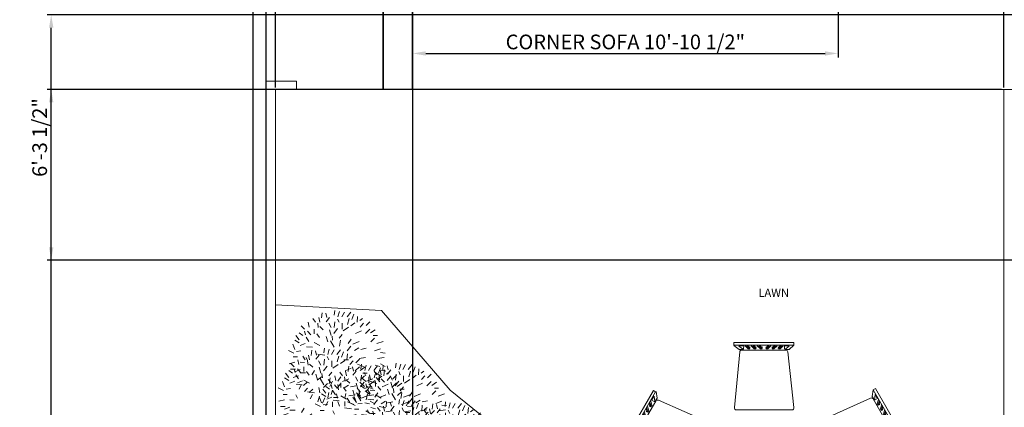
# Model space of a CAD drawing. Units: inches. Extents: x 1239 to 2276906, y 2273 to 321338.
# Tile 5 of 23: x 1239 to 1541, y 2510 to 2629. Entities that reach past the tile are written whole.
import ezdxf

# ---------------------------------------------------------------- set-up
doc = ezdxf.new("R2010")
doc.units = ezdxf.units.IN
for name, color, linetype, lineweight in [('A-ANNO-DIMS', 2, 'Continuous', 18), ('A-AREA-IDEN', 7, 'Continuous', 18), ('A-FURN', 8, 'Continuous', 13), ('C-PROP', 7, 'Continuous', 25), ('L-PLNT', 94, 'Continuous', 13), ('wall', 7, 'Continuous', 35)]:
    doc.layers.add(name, color=color, linetype=linetype, lineweight=lineweight)
doc.styles.get("Standard").update_dxf_attribs({"font": 'arial.ttf'})
doc.dimstyles.new('ISO-25', dxfattribs={"dimtxt": 4.5, "dimasz": 4, "dimexe": 1.25, "dimexo": 0.625, "dimtad": 1, "dimdec": 1, "dimlunit": 3, "dimtxsty": 'Standard', "dimcen": 2.5, "dimadec": 0, "dimazin": 0, "dimtfac": 1, "dimtdec": 1, "dimtmove": 0, "dimatfit": 3, "dimfxl": 1, "dimarcsym": 0})

# ---------------------------------------------------------------- blocks, each defined once
blk = doc.blocks.new('A$C20C17E7E')
for p, q in [((1.807, 4.871), (1.746, 5.147)), ((1.899, 5.117), (1.929, 5.423)), ((2.205, 5.147), (2.144, 5.393)), ((2.174, 4.903), (2.359, 5.147)), ((2.635, 5.271), (2.665, 5.546)), ((2.849, 5.179), (2.941, 5.485)), ((3.063, 5.179), (3.217, 5.455)), ((3.37, 5.179), (3.584, 5.455)), ((3.646, 5.025), (3.768, 5.332)), ((3.952, 4.871), (3.983, 5.21)), ((0.919, 4.474), (0.735, 4.658)), ((1.195, 4.597), (1.134, 4.871)), ((1.562, 4.871), (1.409, 5.086)), ((1.716, 4.565), (1.685, 4.81)), ((1.991, 4.443), (1.807, 4.627)), ((2.45, 4.565), (2.328, 4.81)), ((2.635, 4.565), (2.665, 4.903)), ((2.91, 4.871), (2.819, 5.056)), ((3.095, 4.474), (3.095, 4.81)), ((3.156, 4.382), (3.462, 4.597)), ((3.401, 4.749), (3.492, 5.086)), ((3.584, 4.658), (3.829, 4.841)), ((4.105, 4.964), (4.259, 5.086)), ((4.135, 4.597), (4.32, 4.81)), ((4.472, 4.688), (4.687, 4.903)), ((0.613, 3.861), (0.428, 4.106)), ((0.827, 4.106), (0.613, 4.259)), ((0.98, 4.137), (0.919, 4.352)), ((1.164, 3.77), (1.01, 4.014)), ((1.286, 4.137), (1.102, 4.352)), ((1.47, 4.198), (1.47, 4.474)), ((1.777, 3.983), (1.623, 4.198)), ((2.267, 3.739), (2.174, 4.045)), ((2.45, 4.106), (2.359, 4.443)), ((2.543, 3.831), (2.513, 4.076)), ((2.604, 4.228), (2.819, 4.504)), ((2.91, 3.953), (3.095, 4.167)), ((3.86, 4.228), (4.196, 4.382)), ((4.442, 4.228), (4.687, 4.474)), ((4.717, 4.259), (4.993, 4.443)), ((4.871, 4.106), (5.117, 4.106)), ((0.367, 3.31), (0.244, 3.616)), ((0.613, 3.677), (0.367, 3.831)), ((0.949, 3.646), (0.674, 3.524)), ((1.378, 3.431), (1.041, 3.463)), ((1.807, 3.524), (1.47, 3.707)), ((2.635, 3.431), (2.42, 3.8)), ((2.941, 3.494), (3.002, 3.831)), ((3.37, 3.218), (3.584, 3.494)), ((3.431, 3.646), (3.614, 3.892)), ((3.707, 3.616), (4.074, 3.77)), ((4.748, 3.739), (4.963, 3.953)), ((5.086, 3.646), (5.453, 3.77)), ((0.306, 3.095), (0, 3.249)), ((0.52, 2.88), (0.276, 2.88)), ((0.704, 3.218), (0.459, 3.188)), ((1.102, 2.666), (1.01, 2.849)), ((2.083, 2.973), (1.685, 3.034)), ((3.799, 3.249), (4.044, 3.401)), ((4.074, 2.788), (4.442, 2.849)), ((4.166, 3.31), (4.472, 3.37)), ((4.963, 3.218), (5.3, 3.34)), ((5.117, 2.788), (5.514, 2.849)), ((5.3, 3.125), (5.575, 3.095)), ((0.367, 2.574), (0.03, 2.482)), ((0.919, 2.543), (0.674, 2.574)), ((3.186, 2.697), (3.462, 2.697)), ((3.983, 2.452), (4.35, 2.298)), ((4.993, 2.391), (5.269, 2.33)), ((5.3, 2.482), (5.575, 2.33)), ((0.398, 2.176), (0.122, 2.176)), ((0.582, 1.778), (0.276, 1.685)), ((0.674, 2.145), (0.367, 2.022)), ((0.98, 1.961), (0.674, 1.961)), ((1.501, 2.084), (1.347, 1.839)), ((1.929, 1.748), (1.653, 1.533)), ((5.056, 1.931), (5.3, 1.778)), ((5.331, 2.115), (5.607, 2.054)), ((0.796, 1.502), (0.52, 1.379)), ((0.735, 1.257), (0.613, 1.012)), ((1.071, 1.409), (0.858, 1.226)), ((2.237, 1.348), (2.022, 1.103)), ((2.543, 1.472), (2.389, 1.164)), ((2.849, 1.287), (2.88, 0.981)), ((4.105, 1.409), (4.381, 1.164)), ((4.535, 1.164), (4.871, 1.012)), ((4.687, 1.472), (5.086, 1.348)), ((5.056, 1.685), (5.269, 1.44)), ((1.102, 1.073), (0.919, 0.888)), ((1.409, 1.012), (1.195, 0.827)), ((1.378, 0.705), (1.256, 0.46)), ((1.777, 0.614), (1.685, 0.276)), ((1.746, 1.103), (1.807, 0.797)), ((2.328, 0.827), (2.267, 0.521)), ((2.543, 0.951), (2.45, 0.705)), ((2.757, 0.736), (2.819, 0.491)), ((3.308, 0.766), (3.247, 0.491)), ((4.013, 0.736), (4.166, 0.491)), ((4.411, 0.92), (4.687, 0.705)), ((2.083, 0.521), (1.961, 0.215)), ((2.267, 0.306), (2.144, 0.062)), ((2.543, 0.276), (2.543, 0)), ((2.849, 0.306), (2.941, 0.03)), ((3.247, 0.306), (3.247, 0.03)), ((3.37, 0.491), (3.523, 0.245)), ((3.707, 0.552), (3.922, 0.245))]:
    blk.add_line(p, q)
blk = doc.blocks.new('A$C45501D90')
for p, q in [((-242.2, 1133.5), (224, 1133.5)), ((-242.2, 1112.8), (-242.2, 1133.5)), ((224, 1112.8), (-242.2, 1112.8)), ((-242.2, 1111.2), (-202.3, 1079.2)), ((-203.9, 1106.4), (-165.6, 1108)), ((-168.8, 1080.8), (-203.9, 1106.4)), ((-202.3, 1079.2), (-168.8, 1080.8)), ((161.8, 1076.1), (-181.4, 1076.1)), ((-165.6, 1108), (-167.2, 1085.6)), ((-156, 1109.6), (-132, 1085.6)), ((-119.3, 1085.6), (-143.2, 1108)), ((-143.2, 1108), (-133.6, 1108)), ((-133.6, 1108), (-122.5, 1098.4)), ((-132, 1085.6), (-119.3, 1085.6)), ((-122.5, 1098.4), (-119.3, 1101.6)), ((-119.3, 1101.6), (-117.7, 1087.2)), ((-108.1, 1109.6), (-84.1, 1085.6)), ((-71.4, 1085.6), (-95.3, 1108)), ((-95.3, 1108), (-85.7, 1108)), ((-85.7, 1108), (-74.6, 1098.4)), ((-84.1, 1085.6), (-71.4, 1085.6)), ((-74.6, 1098.4), (-71.4, 1101.6)), ((-71.4, 1101.6), (-69.8, 1087.2)), ((-60.2, 1109.6), (-36.2, 1085.6)), ((-23.5, 1085.6), (-47.4, 1108)), ((-47.4, 1108), (-37.8, 1108)), ((-37.8, 1108), (-26.7, 1098.4)), ((-36.2, 1085.6), (-23.5, 1085.6)), ((-26.7, 1098.4), (-23.5, 1101.6)), ((-23.5, 1101.6), (-21.9, 1087.2)), ((8.5, 1101.6), (6.9, 1087.2)), ((8.5, 1085.6), (32.4, 1108)), ((11.6, 1098.4), (8.5, 1101.6)), ((21.2, 1085.6), (8.5, 1085.6)), ((22.8, 1108), (11.6, 1098.4)), ((45.2, 1109.6), (21.2, 1085.6)), ((32.4, 1108), (22.8, 1108)), ((56.3, 1101.6), (54.8, 1087.2)), ((56.3, 1085.6), (80.3, 1108)), ((59.5, 1098.4), (56.3, 1101.6)), ((69.1, 1085.6), (56.3, 1085.6)), ((70.7, 1108), (59.5, 1098.4)), ((93.1, 1109.6), (69.1, 1085.6)), ((80.3, 1108), (70.7, 1108)), ((104.2, 1101.6), (102.6, 1087.2)), ((104.2, 1085.6), (128.2, 1108)), ((107.4, 1098.4), (104.2, 1101.6)), ((117, 1085.6), (104.2, 1085.6)), ((118.6, 1108), (107.4, 1098.4)), ((141, 1109.6), (117, 1085.6)), ((128.2, 1108), (118.6, 1108)), ((188.9, 1106.4), (150.5, 1108)), ((150.5, 1108), (152.1, 1085.6)), ((153.7, 1080.8), (188.9, 1106.4)), ((187.3, 1079.2), (153.7, 1080.8)), ((224, 1112.8), (187.3, 1079.2)), ((224, 1133.5), (224, 1112.8)), ((-197.3, 1061.6), (-238.9, 627.6)), ((225.2, 627.8), (177.6, 1061.8)), ((842.6, 766.1), (860.5, 776.5)), ((860.5, 776.5), (1093.6, 372.8)), ((-1102.7, 357), (-869.7, 760.7)), ((-851.7, 750.4), (-1084.8, 346.6)), ((-863.7, 716.7), (-884.3, 684.4)), ((-869.7, 760.7), (-851.7, 750.4)), ((-859.2, 673.6), (-863.7, 716.7)), ((-841, 701.8), (-859.2, 673.6)), ((-848.7, 752.3), (-841, 701.8)), ((820.7, 701.7), (424.1, 520.7)), ((841.2, 765.3), (833.5, 714.8)), ((833.5, 714.8), (851.7, 686.6)), ((1012.8, 397.9), (841.2, 695.1)), ((1075.7, 362.4), (842.6, 766.1)), ((851.7, 686.6), (856.2, 729.8)), ((856.2, 729.8), (876.7, 697.4)), ((876.7, 697.4), (856.6, 687.6)), ((-851, 678.1), (-1022.6, 380.9)), ((-919.4, 623.5), (-924.2, 615.2)), ((-924.2, 615.2), (-921.5, 600.8)), ((-912, 591.6), (-919.4, 623.5)), ((-914.4, 635.4), (-905.6, 602.7)), ((-897.5, 642.2), (-901.9, 641.1)), ((-901.9, 641.1), (-890.2, 632.5)), ((-895.4, 665), (-900.2, 656.7)), ((-900.2, 656.7), (-897.5, 642.2)), ((-888.1, 633.1), (-895.4, 665)), ((-890.4, 676.9), (-881.7, 644.2)), ((-881.7, 644.2), (-888.1, 633.1)), ((-884.3, 684.4), (-864.1, 674.6)), ((-431.1, 509), (-830.8, 684.8)), ((882.9, 689.9), (874.2, 657.2)), ((874.2, 657.2), (880.6, 646.1)), ((880.6, 646.1), (887.9, 678)), ((894.4, 654.1), (882.7, 645.5)), ((887.9, 678), (892.7, 669.7)), ((892.7, 669.7), (890, 655.2)), ((890, 655.2), (894.4, 654.1)), ((906.9, 648.4), (898.1, 615.7)), ((898.1, 615.7), (904.5, 604.6)), ((904.5, 604.6), (911.9, 636.5)), ((911.9, 636.5), (916.7, 628.2)), ((916.7, 628.2), (914, 613.8)), ((914, 613.8), (918.3, 612.6)), ((-945.4, 559.3), (-949.8, 558.1)), ((-949.8, 558.1), (-938.1, 549.6)), ((-943.3, 582), (-948.1, 573.8)), ((-948.1, 573.8), (-945.4, 559.3)), ((-936, 550.1), (-943.3, 582)), ((-938.3, 593.9), (-929.6, 561.2)), ((-929.6, 561.2), (-936, 550.1)), ((-921.5, 600.8), (-925.8, 599.6)), ((-925.8, 599.6), (-914.2, 591)), ((-905.6, 602.7), (-912, 591.6)), ((-223, 610.1), (209.4, 610.1)), ((918.3, 612.6), (906.7, 604)), ((930.8, 606.9), (922.1, 574.2)), ((922.1, 574.2), (928.4, 563.1)), ((928.4, 563.1), (935.8, 595.1)), ((942.3, 571.1), (930.6, 562.6)), ((935.8, 595.1), (940.6, 586.8)), ((940.6, 586.8), (937.9, 572.3)), ((937.9, 572.3), (942.3, 571.1)), ((958.2, 543.5), (945, 537.7)), ((957.1, 539.1), (958.2, 543.5)), ((970.9, 534.2), (957.1, 539.1)), ((-1015, 461.2), (-982.3, 469.9)), ((-975.9, 481), (-1007.2, 471.4)), ((-1007.2, 471.4), (-1002.4, 479.7)), ((-1002.4, 479.7), (-988.5, 484.6)), ((-991, 502.7), (-958.3, 511.4)), ((-988.5, 484.6), (-989.7, 489)), ((-989.7, 489), (-976.5, 483.2)), ((-951.9, 522.5), (-983.2, 512.9)), ((-983.2, 512.9), (-978.5, 521.2)), ((-982.3, 469.9), (-975.9, 481)), ((-978.5, 521.2), (-964.6, 526.1)), ((-964.6, 526.1), (-965.7, 530.5)), ((-965.7, 530.5), (-952.5, 524.7)), ((-958.3, 511.4), (-951.9, 522.5)), ((-639.9, 111.9), (-423.7, 486.4)), ((-5.6, 508.7, 90.8), (0.4, 508.7, 90.8)), ((-5.6, 317.7, 90.8), (-5.6, 508.7, 90.8)), ((0.4, 508.7, 90.8), (0.4, 317.7, 90.8)), ((5.8, 317.7, 90.8), (5.8, 508.7, 90.8)), ((5.8, 508.7, 90.8), (11.8, 508.7, 90.8)), ((11.8, 508.7, 90.8), (11.8, 317.7, 90.8)), ((416.9, 498.2), (633.1, 123.7)), ((950.8, 524.4), (944.4, 535.5)), ((944.4, 535.5), (975.7, 525.9)), ((983.5, 515.7), (950.8, 524.4)), ((968.4, 494), (999.7, 484.4)), ((974.7, 483), (968.4, 494)), ((982.2, 502), (968.9, 496.2)), ((975.7, 525.9), (970.9, 534.2)), ((1007.4, 474.2), (974.7, 483)), ((981, 497.6), (982.2, 502)), ((994.9, 492.7), (981, 497.6)), ((1006.1, 460.5), (992.9, 454.7)), ((999.7, 484.4), (994.9, 492.7)), ((1005, 456.2), (1006.1, 460.5)), ((-1060.1, 376.6), (-1042.3, 410.6)), ((-1020.4, 394.3), (-1060.1, 376.6)), ((-1042.3, 410.6), (-1023.8, 398.1)), ((-1038.9, 419.7), (-1006.2, 428.5)), ((-1035.8, 364.4), (-1020.4, 394.3)), ((-999.8, 439.5), (-1031.1, 430)), ((-1031.1, 430), (-1026.3, 438.3)), ((-1026.3, 438.3), (-1012.5, 443.1)), ((-1012.5, 443.1), (-1013.6, 447.5)), ((-1013.6, 447.5), (-1000.4, 441.7)), ((-1006.2, 428.5), (-999.8, 439.5)), ((998.7, 441.5), (992.3, 452.5)), ((992.3, 452.5), (1023.6, 443)), ((1031.4, 432.7), (998.7, 441.5)), ((1018.8, 451.3), (1005, 456.2)), ((1028.3, 377.5), (1012.9, 407.3)), ((1012.9, 407.3), (1052.6, 389.6)), ((1034.8, 423.6), (1016.3, 411.1)), ((1023.6, 443), (1018.8, 451.3)), ((1052.6, 389.6), (1034.8, 423.6)), ((-1084.8, 346.6), (-1102.7, 357)), ((-1083.4, 345.8), (-1035.8, 364.4)), ((-1018, 360), (-663, 106.9)), ((-22.3, 329.1, 90.8), (-22.3, 344.6, 90.8)), ((-22.3, 344.6, 90.8), (-5.6, 344.6, 90.8)), ((-5.6, 329.1, 90.8), (-22.3, 329.1, 90.8)), ((0.4, 317.7, 90.8), (-5.6, 317.7, 90.8)), ((0.4, 344.6, 90.8), (5.8, 344.6, 90.8)), ((5.8, 329.1, 90.8), (0.4, 329.1, 90.8)), ((11.8, 317.7, 90.8), (5.8, 317.7, 90.8)), ((11.8, 344.6, 90.8), (27.3, 344.6, 90.8)), ((27.3, 329.1, 90.8), (11.8, 329.1, 90.8)), ((27.3, 344.6, 90.8), (27.3, 329.1, 90.8)), ((656.3, 118.9), (1008.4, 377.1)), ((1075.9, 358.8), (1028.3, 377.5)), ((1093.6, 372.8), (1075.7, 362.4)), ((-436.3, 265.3, 90.8), (-433.3, 270.5, 90.8)), ((-270.9, 169.9, 90.8), (-436.3, 265.3, 90.8)), ((-433.3, 270.5, 90.8), (-267.9, 175, 90.8)), ((-430.6, 275.2, 90.8), (-427.6, 280.3, 90.8)), ((-265.2, 179.7, 90.8), (-430.6, 275.2, 90.8)), ((-427.6, 280.3, 90.8), (-262.3, 184.9, 90.8)), ((-175.3, 276.1, 90.8), (-104.8, 293.2, 90.8)), ((-103.3, 252.4, 90.8), (-175.3, 276.1, 90.8)), ((-104.8, 293.2, 90.8), (-85.5, 278.4, 90.8)), ((-59.5, 246.5, 90.8), (-103.3, 252.4, 90.8)), ((-85.5, 278.4, 90.8), (-52.1, 293.9, 90.8)), ((9.5, 276.1, 90.8), (-59.5, 246.5, 90.8)), ((-52.1, 293.9, 90.8), (9.5, 276.1, 90.8)), ((134.3, 288, 90.8), (184.3, 235.5, 90.8)), ((149.7, 213.9, 90.8), (134.3, 288, 90.8)), ((184.3, 235.5, 90.8), (181.1, 211.4, 90.8)), ((255.2, 161.9, 90.8), (420.6, 257.3, 90.8)), ((423.5, 252.2, 90.8), (258.2, 156.7, 90.8)), ((260.9, 152, 90.8), (426.2, 247.5, 90.8)), ((429.2, 242.3, 90.8), (263.8, 146.9, 90.8)), ((420.6, 257.3, 90.8), (423.5, 252.2, 90.8)), ((426.2, 247.5, 90.8), (429.2, 242.3, 90.8)), ((-302.5, 168.8, 90.8), (-294.2, 183.3, 90.8)), ((-289.1, 161.1, 90.8), (-302.5, 168.8, 90.8)), ((-291.2, 188.5, 90.8), (-288.5, 193.1, 90.8)), ((-280.7, 175.5, 90.8), (-289.1, 161.1, 90.8)), ((-285.5, 198.3, 90.8), (-277.8, 211.7, 90.8)), ((-277.8, 211.7, 90.8), (-264.3, 204, 90.8)), ((-275.1, 185.4, 90.8), (-277.8, 180.7, 90.8)), ((-273.6, 117.6, 90.8), (-227.4, 162.1, 90.8)), ((-264.3, 204, 90.8), (-272.1, 190.5, 90.8)), ((-267.9, 175, 90.8), (-270.9, 169.9, 90.8)), ((-262.3, 184.9, 90.8), (-265.2, 179.7, 90.8)), ((-227.4, 162.1, 90.8), (-236.2, 87.5, 90.8)), ((166.5, 173, 90.8), (149.7, 213.9, 90.8)), ((226.7, 128.1, 90.8), (166.5, 173, 90.8)), ((181.1, 211.4, 90.8), (211.3, 190.3, 90.8)), ((211.3, 190.3, 90.8), (226.7, 128.1, 90.8)), ((258.2, 156.7, 90.8), (255.2, 161.9, 90.8)), ((256.6, 182, 90.8), (270.1, 189.8, 90.8)), ((265, 167.5, 90.8), (256.6, 182, 90.8)), ((270.7, 157.7, 90.8), (268, 162.4, 90.8)), ((270.1, 189.8, 90.8), (278.4, 175.3, 90.8)), ((281.4, 170.1, 90.8), (284.1, 165.5, 90.8)), ((287.1, 160.3, 90.8), (294.9, 146.8, 90.8)), ((-299.3, 71.7, 90.8), (-276.8, 80.9, 90.8)), ((-276.8, 80.9, 90.8), (-273.6, 117.6, 90.8)), ((-236.2, 87.5, 90.8), (-263.2, 52.5, 90.8)), ((263.8, 146.9, 90.8), (260.9, 152, 90.8)), ((281.4, 139.1, 90.8), (273.7, 152.5, 90.8)), ((294.9, 146.8, 90.8), (281.4, 139.1, 90.8)), ((-319.8, 2.1, 90.8), (-299.3, 71.7, 90.8)), ((-263.2, 52.5, 90.8), (-319.8, 2.1, 90.8)), ((242.9, -24.6, 90.8), (299.4, 25.9, 90.8)), ((299.4, 25.9, 90.8), (278.9, -43.7, 90.8)), ((207, -134.1, 90.8), (215.8, -59.5, 90.8)), ((215.8, -59.5, 90.8), (242.9, -24.6, 90.8)), ((256.4, -53, 90.8), (253.2, -89.7, 90.8)), ((278.9, -43.7, 90.8), (256.4, -53, 90.8)), ((-656.3, -118.9), (-1008.4, -377.1)), ((-416.9, -498.2), (-633.1, -123.7)), ((-449.6, -214.4, 90.8), (-284.2, -118.9, 90.8)), ((-281.2, -124.1, 90.8), (-446.6, -219.5, 90.8)), ((-443.9, -224.2, 90.8), (-278.5, -128.7, 90.8)), ((-275.5, -133.9, 90.8), (-440.9, -229.4, 90.8)), ((-315.2, -118.9, 90.8), (-301.8, -111.1, 90.8)), ((-307.5, -132.3, 90.8), (-315.2, -118.9, 90.8)), ((-301.8, -142.1, 90.8), (-304.5, -137.5, 90.8)), ((-301.8, -111.1, 90.8), (-294, -124.6, 90.8)), ((-290.4, -161.8, 90.8), (-298.8, -147.3, 90.8)), ((-291, -129.7, 90.8), (-288.3, -134.4, 90.8)), ((-285.4, -139.5, 90.8), (-277, -154, 90.8)), ((-284.2, -118.9, 90.8), (-281.2, -124.1, 90.8)), ((-278.5, -128.7, 90.8), (-275.5, -133.9, 90.8)), ((-247, -100.1, 90.8), (-186.8, -145, 90.8)), ((-231.7, -162.3, 90.8), (-247, -100.1, 90.8)), ((-186.8, -145, 90.8), (-170.1, -185.9, 90.8)), ((253.2, -89.7, 90.8), (207, -134.1, 90.8)), ((241.9, -156.9, 90.8), (244.9, -151.7, 90.8)), ((244.9, -151.7, 90.8), (410.3, -247.2, 90.8)), ((247.6, -147.1, 90.8), (250.6, -141.9, 90.8)), ((413, -242.5, 90.8), (247.6, -147.1, 90.8)), ((250.6, -141.9, 90.8), (415.9, -237.4, 90.8)), ((254.7, -157.4, 90.8), (257.4, -152.7, 90.8)), ((260.4, -147.6, 90.8), (268.7, -133.1, 90.8)), ((268.7, -133.1, 90.8), (282.2, -140.8, 90.8)), ((282.2, -140.8, 90.8), (273.8, -155.3, 90.8)), ((639.9, -111.9), (423.7, -486.4)), ((1018, -360), (663, -106.9)), ((-446.6, -219.5, 90.8), (-449.6, -214.4, 90.8)), ((-440.9, -229.4, 90.8), (-443.9, -224.2, 90.8)), ((-277, -154, 90.8), (-290.4, -161.8, 90.8)), ((-201.5, -183.4, 90.8), (-231.7, -162.3, 90.8)), ((-204.7, -207.6, 90.8), (-201.5, -183.4, 90.8)), ((-154.7, -260.1, 90.8), (-204.7, -207.6, 90.8)), ((-170.1, -185.9, 90.8), (-154.7, -260.1, 90.8)), ((-29.8, -248.2, 90.8), (39.2, -218.5, 90.8)), ((39.2, -218.5, 90.8), (83, -224.4, 90.8)), ((83, -224.4, 90.8), (154.9, -248.2, 90.8)), ((407.3, -252.4, 90.8), (241.9, -156.9, 90.8)), ((244, -176, 90.8), (251.7, -162.5, 90.8)), ((257.4, -183.7, 90.8), (244, -176, 90.8)), ((265.2, -170.3, 90.8), (257.4, -183.7, 90.8)), ((270.8, -160.5, 90.8), (268.1, -165.1, 90.8)), ((-47.6, -316.6, 90.8), (-47.6, -301.1, 90.8)), ((-47.6, -301.1, 90.8), (-32.1, -301.1, 90.8)), ((-32.1, -480.7, 90.8), (-32.1, -289.8, 90.8)), ((-32.1, -289.8, 90.8), (-26.1, -289.8, 90.8)), ((31.8, -266, 90.8), (-29.8, -248.2, 90.8)), ((-26.1, -289.8, 90.8), (-26.1, -480.7, 90.8)), ((-26.1, -301.1, 90.8), (-20.8, -301.1, 90.8)), ((-20.8, -480.7, 90.8), (-20.8, -289.8, 90.8)), ((-20.8, -289.8, 90.8), (-14.8, -289.8, 90.8)), ((-14.8, -289.8, 90.8), (-14.8, -480.7, 90.8)), ((-14.8, -301.1, 90.8), (1.9, -301.1, 90.8)), ((1.9, -301.1, 90.8), (1.9, -316.6, 90.8)), ((65.2, -250.4, 90.8), (31.8, -266, 90.8)), ((84.4, -265.2, 90.8), (65.2, -250.4, 90.8)), ((154.9, -248.2, 90.8), (84.4, -265.2, 90.8)), ((410.3, -247.2, 90.8), (407.3, -252.4, 90.8)), ((415.9, -237.4, 90.8), (413, -242.5, 90.8)), ((-1093.6, -372.8), (-1075.7, -362.4)), ((-860.5, -776.5), (-1093.6, -372.8)), ((-1075.9, -358.8), (-1028.3, -377.5)), ((-1075.7, -362.4), (-842.6, -766.1)), ((-1028.3, -377.5), (-1012.9, -407.3)), ((-32.1, -316.6, 90.8), (-47.6, -316.6, 90.8)), ((-20.8, -316.6, 90.8), (-26.1, -316.6, 90.8)), ((1.9, -316.6, 90.8), (-14.8, -316.6, 90.8)), ((851, -678.1), (1022.6, -380.9)), ((851.7, -750.4), (1084.8, -346.6)), ((1102.7, -357), (869.7, -760.7)), ((1035.8, -364.4), (1020.4, -394.3)), ((1020.4, -394.3), (1060.1, -376.6)), ((1083.4, -345.8), (1035.8, -364.4)), ((1060.1, -376.6), (1042.3, -410.6)), ((1084.8, -346.6), (1102.7, -357)), ((-1052.6, -389.6), (-1034.8, -423.6)), ((-1012.9, -407.3), (-1052.6, -389.6)), ((-1034.8, -423.6), (-1016.3, -411.1)), ((-1031.4, -432.7), (-998.7, -441.5)), ((-1023.6, -443), (-1018.8, -451.3)), ((-992.3, -452.5), (-1023.6, -443)), ((-1018.8, -451.3), (-1005, -456.2)), ((-1012.8, -397.9), (-841.2, -695.1)), ((-1006.1, -460.5), (-992.9, -454.7)), ((-1005, -456.2), (-1006.1, -460.5)), ((-998.7, -441.5), (-992.3, -452.5)), ((1006.2, -428.5), (999.8, -439.5)), ((999.8, -439.5), (1031.1, -430)), ((1013.6, -447.5), (1000.4, -441.7)), ((1038.9, -419.7), (1006.2, -428.5)), ((1026.3, -438.3), (1012.5, -443.1)), ((1012.5, -443.1), (1013.6, -447.5)), ((1042.3, -410.6), (1023.8, -398.1)), ((1031.1, -430), (1026.3, -438.3)), ((-1007.4, -474.2), (-974.7, -483)), ((-968.4, -494), (-999.7, -484.4)), ((-999.7, -484.4), (-994.9, -492.7)), ((-994.9, -492.7), (-981, -497.6)), ((-983.5, -515.7), (-950.8, -524.4)), ((-982.2, -502), (-968.9, -496.2)), ((-981, -497.6), (-982.2, -502)), ((-944.4, -535.5), (-975.7, -525.9)), ((-975.7, -525.9), (-970.9, -534.2)), ((-974.7, -483), (-968.4, -494)), ((-970.9, -534.2), (-957.1, -539.1)), ((-950.8, -524.4), (-944.4, -535.5)), ((-820.7, -701.7), (-424.1, -520.7)), ((-26.1, -480.7, 90.8), (-32.1, -480.7, 90.8)), ((-14.8, -480.7, 90.8), (-20.8, -480.7, 90.8)), ((431.1, -509), (830.8, -684.8)), ((958.3, -511.4), (951.9, -522.5)), ((951.9, -522.5), (983.2, -512.9)), ((965.7, -530.5), (952.5, -524.7)), ((991, -502.7), (958.3, -511.4)), ((978.5, -521.2), (964.6, -526.1)), ((964.6, -526.1), (965.7, -530.5)), ((982.3, -469.9), (975.9, -481)), ((975.9, -481), (1007.2, -471.4)), ((989.7, -489), (976.5, -483.2)), ((983.2, -512.9), (978.5, -521.2)), ((1015, -461.2), (982.3, -469.9)), ((1002.4, -479.7), (988.5, -484.6)), ((988.5, -484.6), (989.7, -489)), ((1007.2, -471.4), (1002.4, -479.7)), ((-958.2, -543.5), (-945, -537.7)), ((-957.1, -539.1), (-958.2, -543.5)), ((-942.3, -571.1), (-930.6, -562.6)), ((-937.9, -572.3), (-942.3, -571.1)), ((-940.6, -586.8), (-937.9, -572.3)), ((-935.8, -595.1), (-940.6, -586.8)), ((-928.4, -563.1), (-935.8, -595.1)), ((-930.8, -606.9), (-922.1, -574.2)), ((-922.1, -574.2), (-928.4, -563.1)), ((-918.3, -612.6), (-906.7, -604)), ((-914, -613.8), (-918.3, -612.6)), ((-904.5, -604.6), (-911.9, -636.5)), ((-898.1, -615.7), (-904.5, -604.6)), ((218.9, -611.6), (-213.5, -611.6)), ((223, -610.1), (-209.4, -610.1)), ((905.6, -602.7), (912, -591.6)), ((914.4, -635.4), (905.6, -602.7)), ((912, -591.6), (919.4, -623.5)), ((925.8, -599.6), (914.2, -591)), ((921.5, -600.8), (925.8, -599.6)), ((924.2, -615.2), (921.5, -600.8)), ((929.6, -561.2), (936, -550.1)), ((938.3, -593.9), (929.6, -561.2)), ((936, -550.1), (943.3, -582)), ((949.8, -558.1), (938.1, -549.6)), ((943.3, -582), (948.1, -573.8)), ((945.4, -559.3), (949.8, -558.1)), ((948.1, -573.8), (945.4, -559.3)), ((-916.7, -628.2), (-914, -613.8)), ((-911.9, -636.5), (-916.7, -628.2)), ((-906.9, -648.4), (-898.1, -615.7)), ((-894.4, -654.1), (-882.7, -645.5)), ((-890, -655.2), (-894.4, -654.1)), ((-892.7, -669.7), (-890, -655.2)), ((-887.9, -678), (-892.7, -669.7)), ((-880.6, -646.1), (-887.9, -678)), ((-882.9, -689.9), (-874.2, -657.2)), ((-874.2, -657.2), (-880.6, -646.1)), ((-876.7, -697.4), (-856.6, -687.6)), ((-851.7, -686.6), (-856.2, -729.8)), ((-833.5, -714.8), (-851.7, -686.6)), ((-229.3, -629.3), (-181.8, -1063.3)), ((-225.2, -627.8), (-177.6, -1061.8)), ((193.2, -1063.1), (234.8, -629.1)), ((197.3, -1061.6), (238.9, -627.6)), ((841, -701.8), (859.2, -673.6)), ((859.2, -673.6), (863.7, -716.7)), ((863.7, -716.7), (884.3, -684.4)), ((884.3, -684.4), (864.1, -674.6)), ((881.7, -644.2), (888.1, -633.1)), ((890.4, -676.9), (881.7, -644.2)), ((888.1, -633.1), (895.4, -665)), ((901.9, -641.1), (890.2, -632.5)), ((895.4, -665), (900.2, -656.7)), ((897.5, -642.2), (901.9, -641.1)), ((900.2, -656.7), (897.5, -642.2)), ((919.4, -623.5), (924.2, -615.2)), ((-856.2, -729.8), (-876.7, -697.4)), ((-842.6, -766.1), (-860.5, -776.5)), ((-841.2, -765.3), (-833.5, -714.8)), ((848.7, -752.3), (841, -701.8)), ((869.7, -760.7), (851.7, -750.4)), ((-231.3, -1112.7), (-191.4, -1080.8)), ((-228.1, -1114.3), (238.1, -1114.3)), ((-228.1, -1135), (-228.1, -1114.3)), ((238.1, -1135), (-228.1, -1135)), ((-227.2, -1111.2), (-187.3, -1079.2)), ((-224, -1112.8), (242.2, -1112.8)), ((-224, -1133.5), (-224, -1112.8)), ((242.2, -1133.5), (-224, -1133.5)), ((-157.9, -1082.4), (-193, -1107.9)), ((-193, -1107.9), (-154.7, -1109.5)), ((-191.4, -1080.8), (-157.9, -1082.4)), ((-153.7, -1080.8), (-188.9, -1106.4)), ((-188.9, -1106.4), (-150.5, -1108)), ((-187.3, -1079.2), (-153.7, -1080.8)), ((-165.9, -1077.6), (177.3, -1077.6)), ((-161.8, -1076.1), (181.4, -1076.1)), ((-154.7, -1109.5), (-156.3, -1087.1)), ((-150.5, -1108), (-152.1, -1085.6)), ((-145.1, -1111.1), (-121.1, -1087.1)), ((-141, -1109.6), (-117, -1085.6)), ((-108.4, -1087.1), (-132.3, -1109.5)), ((-132.3, -1109.5), (-122.7, -1109.5)), ((-104.2, -1085.6), (-128.2, -1108)), ((-128.2, -1108), (-118.6, -1108)), ((-122.7, -1109.5), (-111.6, -1099.9)), ((-121.1, -1087.1), (-108.4, -1087.1)), ((-118.6, -1108), (-107.4, -1098.4)), ((-117, -1085.6), (-104.2, -1085.6)), ((-111.6, -1099.9), (-108.4, -1103.1)), ((-108.4, -1103.1), (-106.8, -1088.7)), ((-107.4, -1098.4), (-104.2, -1101.6)), ((-104.2, -1101.6), (-102.6, -1087.2)), ((-97.2, -1111.1), (-73.2, -1087.1)), ((-93.1, -1109.6), (-69.1, -1085.6)), ((-60.5, -1087.1), (-84.4, -1109.5)), ((-84.4, -1109.5), (-74.8, -1109.5)), ((-56.3, -1085.6), (-80.3, -1108)), ((-80.3, -1108), (-70.7, -1108)), ((-74.8, -1109.5), (-63.7, -1099.9)), ((-73.2, -1087.1), (-60.5, -1087.1)), ((-70.7, -1108), (-59.5, -1098.4)), ((-69.1, -1085.6), (-56.3, -1085.6)), ((-63.7, -1099.9), (-60.5, -1103.1)), ((-60.5, -1103.1), (-58.9, -1088.7)), ((-59.5, -1098.4), (-56.3, -1101.6)), ((-56.3, -1101.6), (-54.8, -1087.2)), ((-49.3, -1111.1), (-25.3, -1087.1)), ((-45.2, -1109.6), (-21.2, -1085.6)), ((-12.6, -1087.1), (-36.5, -1109.5)), ((-36.5, -1109.5), (-26.9, -1109.5)), ((-8.5, -1085.6), (-32.4, -1108)), ((-32.4, -1108), (-22.8, -1108)), ((-26.9, -1109.5), (-15.8, -1099.9)), ((-25.3, -1087.1), (-12.6, -1087.1)), ((-22.8, -1108), (-11.6, -1098.4)), ((-21.2, -1085.6), (-8.5, -1085.6)), ((-15.8, -1099.9), (-12.6, -1103.1)), ((-12.6, -1103.1), (-11, -1088.7)), ((-11.6, -1098.4), (-8.5, -1101.6)), ((-8.5, -1101.6), (-6.9, -1087.2)), ((19.4, -1103.1), (17.8, -1088.7)), ((19.4, -1087.1), (43.3, -1109.5)), ((32.1, -1087.1), (19.4, -1087.1)), ((22.6, -1099.9), (19.4, -1103.1)), ((23.5, -1101.6), (21.9, -1087.2)), ((33.7, -1109.5), (22.6, -1099.9)), ((23.5, -1085.6), (47.4, -1108)), ((36.2, -1085.6), (23.5, -1085.6)), ((26.7, -1098.4), (23.5, -1101.6)), ((37.8, -1108), (26.7, -1098.4)), ((56.1, -1111.1), (32.1, -1087.1)), ((43.3, -1109.5), (33.7, -1109.5)), ((60.2, -1109.6), (36.2, -1085.6)), ((47.4, -1108), (37.8, -1108)), ((67.3, -1103.1), (65.7, -1088.7)), ((67.3, -1087.1), (91.2, -1109.5)), ((80, -1087.1), (67.3, -1087.1)), ((70.4, -1099.9), (67.3, -1103.1)), ((71.4, -1101.6), (69.8, -1087.2)), ((81.6, -1109.5), (70.4, -1099.9)), ((71.4, -1085.6), (95.3, -1108)), ((84.1, -1085.6), (71.4, -1085.6)), ((74.6, -1098.4), (71.4, -1101.6)), ((85.7, -1108), (74.6, -1098.4)), ((104, -1111.1), (80, -1087.1)), ((91.2, -1109.5), (81.6, -1109.5)), ((108.1, -1109.6), (84.1, -1085.6)), ((95.3, -1108), (85.7, -1108)), ((115.1, -1103.1), (113.6, -1088.7)), ((115.1, -1087.1), (139.1, -1109.5)), ((127.9, -1087.1), (115.1, -1087.1)), ((118.3, -1099.9), (115.1, -1103.1)), ((119.3, -1101.6), (117.7, -1087.2)), ((129.5, -1109.5), (118.3, -1099.9)), ((119.3, -1085.6), (143.2, -1108)), ((132, -1085.6), (119.3, -1085.6)), ((122.5, -1098.4), (119.3, -1101.6)), ((133.6, -1108), (122.5, -1098.4)), ((151.9, -1111.1), (127.9, -1087.1)), ((139.1, -1109.5), (129.5, -1109.5)), ((156, -1109.6), (132, -1085.6)), ((143.2, -1108), (133.6, -1108)), ((161.4, -1109.5), (163, -1087.1)), ((199.8, -1107.9), (161.4, -1109.5)), ((198.2, -1080.8), (164.6, -1082.4)), ((164.6, -1082.4), (199.8, -1107.9)), ((165.6, -1108), (167.2, -1085.6)), ((203.9, -1106.4), (165.6, -1108)), ((202.3, -1079.2), (168.8, -1080.8)), ((168.8, -1080.8), (203.9, -1106.4)), ((238.1, -1112.7), (198.2, -1080.8)), ((242.2, -1111.2), (202.3, -1079.2)), ((238.1, -1114.3), (238.1, -1135)), ((242.2, -1112.8), (242.2, -1133.5))]:
    blk.add_line(p, q)
for centre, radius in [((0, 0), 537), ((0, 0), 527), ((-94.8, 394.7, 90.8), 61.3), ((96.9, 390, 90.8), 56.9), ((95.5, 390.7, 90.8), 29.4), ((-282.3, 294.7, 90.8), 56.9), ((-283.5, 293.9, 90.8), 29.4), ((277.2, 277.6, 90.8), 61.3), ((-382.1, 131.1, 90.8), 61.3), ((369, 109.3, 90.8), 56.9), ((368.9, 110.8, 90.8), 29.4), ((-389.3, -81.3, 90.8), 56.9), ((-389.2, -82.8, 90.8), 29.4), ((361.8, -103.1, 90.8), 61.3), ((-297.5, -249.6, 90.8), 61.3), ((261.9, -266.7, 90.8), 56.9), ((-117.2, -362, 90.8), 56.9), ((74.4, -366.7, 90.8), 61.3), ((263.2, -265.9, 90.8), 29.4), ((-115.9, -362.7, 90.8), 29.4)]:
    blk.add_circle(centre, radius)
for centre, radius, start, end in [((-181.4, 1060.1), 16, 90, 174.51988), ((161.8, 1060.1), 16, 6.25717, 90), ((827.4, 687.1), 16, 30, 114.51988), ((-837.2, 670.1), 16, 66.25717, 150), ((-223, 626.1), 16, 174.51988, 270), ((209.4, 626.1), 16, 270, 6.25717), ((-437.5, 494.4), 16, 330, 66.25717), ((430.7, 506.2), 16, 114.51988, 210), ((999, 389.9), 16, 306.25717, 30), ((-1008.8, 373), 16, 150, 234.51988), ((-77.3, 270.2, 90.8), 44.6, 25.85584, 153.33587), ((-77.3, 270.2, 90.8), 44.6, 195.93383, 342.9389), ((178.1, 200.3, 90.8), 44.6, 135.93383, 282.9389), ((178.1, 200.3, 90.8), 44.6, 325.85584, 93.33587), ((-653.7, 119.9), 16, 234.51988, 330), ((-265.7, 83.9, 90.8), 44.6, 85.85584, 213.33587), ((-265.7, 83.9, 90.8), 44.6, 255.93383, 42.9389), ((646.9, 131.7), 16, 210, 306.25717), ((245.3, -55.9, 90.8), 44.6, 75.93383, 222.9389), ((245.3, -55.9, 90.8), 44.6, 265.85584, 33.33587), ((-646.9, -131.7), 16, 30, 126.25717), ((-198.5, -172.3, 90.8), 44.6, 145.85584, 273.33587), ((-198.5, -172.3, 90.8), 44.6, 315.93383, 102.9389), ((653.7, -119.9), 16, 54.51988, 150), ((57, -242.2, 90.8), 44.6, 15.93383, 162.9389), ((57, -242.2, 90.8), 44.6, 205.85584, 333.33587), ((-999, -389.9), 16, 126.25717, 210), ((1008.8, -373), 16, 330, 54.51988), ((-430.7, -506.2), 16, 294.51988, 30), ((437.5, -494.4), 16, 150, 246.25717), ((-213.5, -627.6), 16, 90, 186.25717), ((-209.4, -626.1), 16, 90, 186.25717), ((218.9, -627.6), 16, 354.51988, 90), ((223, -626.1), 16, 354.51988, 90), ((837.2, -670.1), 16, 246.25717, 330), ((-827.4, -687.1), 16, 210, 294.51988), ((-165.9, -1061.6), 16, 186.25717, 270), ((-161.8, -1060.1), 16, 186.25717, 270), ((177.3, -1061.6), 16, 270, 354.51988), ((181.4, -1060.1), 16, 270, 354.51988)]:
    blk.add_arc(centre, radius, start, end)
blk = doc.blocks.new('*D62')
at = {"layer": 'A-ANNO-DIMS', "color": 0, "lineweight": -2, "transparency": 16777216}
for p, q in [((1359.38, 2637.47), (1359.38, 2617.29)), ((1489.78, 2637.47), (1489.78, 2617.29)), ((1363.38, 2618.54), (1485.78, 2618.54))]:
    blk.add_line(p, q, dxfattribs=at)
at = {"layer": 'A-ANNO-DIMS', "color": 0, "transparency": 16777216}
for points in [[(1363.38, 2619.2), (1363.38, 2617.87), (1359.38, 2618.54)], [(1485.78, 2619.2), (1485.78, 2617.87), (1489.78, 2618.54)]]:
    blk.add_solid(points, dxfattribs=at)
at = {"layer": 'Defpoints', "color": 0, "transparency": 16777216}
for p in [(1359.38, 2638.1), (1489.78, 2638.1), (1489.78, 2618.54)]:
    blk.add_point(p, dxfattribs=at)
at = {"layer": 'A-ANNO-DIMS', "color": 0, "transparency": 16777216, "insert": (1424.58, 2621.49), "char_height": 4.5, "attachment_point": 5}
blk.add_mtext('CORNER SOFA 10\'-10 1/2"', dxfattribs=at)
blk = doc.blocks.new('*D89')
at = {"layer": 'A-ANNO-DIMS', "color": 0, "lineweight": -2, "transparency": 16777216}
for p, q in [((1359.38, 3215.77), (1359.38, 2275.7)), ((1551.38, 3215.77), (1551.38, 2275.7)), ((1363.38, 2276.95), (1547.38, 2276.95))]:
    blk.add_line(p, q, dxfattribs=at)
at = {"layer": 'A-ANNO-DIMS', "color": 0, "transparency": 16777216}
for points in [[(1363.38, 2277.61), (1363.38, 2276.28), (1359.38, 2276.95)], [(1547.38, 2277.61), (1547.38, 2276.28), (1551.38, 2276.95)]]:
    blk.add_solid(points, dxfattribs=at)
at = {"layer": 'Defpoints', "color": 0, "transparency": 16777216}
for p in [(1359.38, 3216.4), (1551.38, 3216.4), (1551.38, 2276.95)]:
    blk.add_point(p, dxfattribs=at)
at = {"layer": 'A-ANNO-DIMS', "color": 0, "transparency": 16777216, "insert": (1455.38, 2279.87), "char_height": 4.5, "attachment_point": 5}
blk.add_mtext('16\'-0"', dxfattribs=at)
blk = doc.blocks.new('*D100')
at = {"layer": 'A-ANNO-DIMS', "color": 0, "lineweight": -2, "transparency": 16777216}
for p, q in [((1550.76, 2630.4), (1247.33, 2630.4)), ((1248.58, 2559.13), (1248.58, 2626.4)), ((1550.76, 2555.13), (1247.33, 2555.13))]:
    blk.add_line(p, q, dxfattribs=at)
at = {"layer": 'A-ANNO-DIMS', "color": 0, "transparency": 16777216}
for points in [[(1247.92, 2626.4), (1249.25, 2626.4), (1248.58, 2630.4)], [(1247.92, 2559.13), (1249.25, 2559.13), (1248.58, 2555.13)]]:
    blk.add_solid(points, dxfattribs=at)
at = {"layer": 'Defpoints', "color": 0, "transparency": 16777216}
for p in [(1248.58, 2630.4), (1551.38, 2630.4), (1551.38, 2555.13)]:
    blk.add_point(p, dxfattribs=at)
at = {"layer": 'A-ANNO-DIMS', "color": 0, "transparency": 16777216, "insert": (1245.63, 2592.76), "char_height": 4.5, "attachment_point": 5, "rotation": 90}
blk.add_mtext('6\'-3 1/2"', dxfattribs=at)
blk = doc.blocks.new('*D102')
at = {"layer": 'A-ANNO-DIMS', "color": 0, "lineweight": -2, "transparency": 16777216}
for p, q in [((1317.38, 2608.14), (1317.38, 3608.95)), ((1321.38, 3607.7), (1536.55, 3607.7)), ((1540.55, 2608.14), (1540.55, 3608.95))]:
    blk.add_line(p, q, dxfattribs=at)
at = {"layer": 'A-ANNO-DIMS', "color": 0, "transparency": 16777216}
for points in [[(1321.38, 3608.36), (1321.38, 3607.03), (1317.38, 3607.7)], [(1536.55, 3608.36), (1536.55, 3607.03), (1540.55, 3607.7)]]:
    blk.add_solid(points, dxfattribs=at)
at = {"layer": 'Defpoints', "color": 0, "transparency": 16777216}
for p in [(1540.55, 3607.7), (1317.38, 2607.52), (1540.55, 2607.52)]:
    blk.add_point(p, dxfattribs=at)
at = {"layer": 'A-ANNO-DIMS', "color": 0, "transparency": 16777216, "insert": (1428.97, 3610.62), "char_height": 4.5, "attachment_point": 5}
blk.add_mtext('18\'-7"', dxfattribs=at)
blk = doc.blocks.new('*D103')
at = {"layer": 'A-ANNO-DIMS', "color": 0, "lineweight": -2, "transparency": 16777216}
for p, q in [((1539.93, 2607.52), (1247.33, 2607.52)), ((1248.58, 2353.9), (1248.58, 2603.52)), ((1539.93, 2349.9), (1247.33, 2349.9))]:
    blk.add_line(p, q, dxfattribs=at)
at = {"layer": 'A-ANNO-DIMS', "color": 0, "transparency": 16777216}
for points in [[(1247.92, 2603.52), (1249.25, 2603.52), (1248.58, 2607.52)], [(1247.92, 2353.9), (1249.25, 2353.9), (1248.58, 2349.9)]]:
    blk.add_solid(points, dxfattribs=at)
at = {"layer": 'Defpoints', "color": 0, "transparency": 16777216}
for p in [(1248.58, 2607.52), (1540.55, 2607.52), (1540.55, 2349.9)]:
    blk.add_point(p, dxfattribs=at)
at = {"layer": 'A-ANNO-DIMS', "color": 0, "transparency": 16777216, "insert": (1245.63, 2478.71), "char_height": 4.5, "attachment_point": 5, "rotation": 90}
blk.add_mtext('21\'-5 1/2"', dxfattribs=at)

msp = doc.modelspace()

# ---------------------------------------------------------------- linework, layer by layer
at = {"layer": 'C-PROP'}
msp.add_line((1314.38, 2607.52), (1314.38, 2349.9), dxfattribs=at)
for points in [[(1970.38, 2345.9), (1970.38, 3545.9), (1310.38, 3545.9), (1310.38, 2345.9), (1644.79, 2345.9)], [(1966.38, 2349.9), (1966.38, 3541.9), (1314.38, 3541.9), (1314.38, 2607.52)]]:
    msp.add_lwpolyline(points, dxfattribs=at)
at = {"layer": 'L-PLNT'}
for p, q in [((1314.38, 2610.07), (1323.74, 2610.07)), ((1323.74, 2610.07), (1323.74, 2607.52)), ((1317.38, 2607.52), (1543.55, 2607.52)), ((1317.38, 2607.52), (1317.38, 2349.9)), ((1540.55, 2607.52), (1540.55, 2349.9))]:
    msp.add_line(p, q, dxfattribs=at)
msp.add_lwpolyline([(1317.38, 2541.46), (1349.79, 2539.69), (1370.85, 2515.28), (1382.64, 2505.8), (1401.64, 2477.52), (1419.31, 2409.19), (1419.31, 2382.63), (1406.62, 2349.9)], dxfattribs=at)
at = {"layer": 'wall'}
for p, q in [((1350.38, 3505.9), (1350.38, 2607.52)), ((1359.38, 3211.9), (1359.38, 2607.52))]:
    msp.add_line(p, q, dxfattribs=at)

# ---------------------------------------------------------------- block references
at = {"layer": 'A-FURN', "xscale": 0.0393700787401575, "yscale": 0.0393700787401575, "zscale": 0.0393700787401575}
msp.add_blockref('A$C45501D90', (1467.4, 2485.22), dxfattribs=at)
at = {"layer": 'L-PLNT', "xscale": 5.31977792485371, "yscale": 5.31977792485371, "zscale": 5.31977792485371}
for p in [(1321.33, 2510.19), (1318.17, 2498.67), (1329.52, 2493.77), (1340.12, 2494.09), (1341.13, 2482.94), (1355.28, 2482.2)]:
    msp.add_blockref('A$C20C17E7E', p, dxfattribs=at)

# ---------------------------------------------------------------- texts
at = {"layer": 'A-AREA-IDEN', "insert": (1465.36, 2546.4), "char_height": 2.5, "attachment_point": 1}
msp.add_mtext_dynamic_manual_height_columns('LAWN ', width=44.9462, gutter_width=12.5, heights=[0], dxfattribs=at)

# ---------------------------------------------------------------- dimensions: what is measured, and where the dimension line sits
at = {"layer": 'A-ANNO-DIMS'}
for base, p1, p2, picture, middle in [((1540.55, 3607.7), (1317.38, 2607.52), (1540.55, 2607.52), '*D102', (1428.97, 3610.62)), ((1551.38, 2276.95), (1359.38, 3216.4), (1551.38, 3216.4), '*D89', (1455.38, 2279.87))]:
    dim = msp.add_linear_dim(base=base, p1=p1, p2=p2, dimstyle='ISO-25', override={"dimdec": 1, "dimlfac": 1, "dimrnd": 0, "dimzin": 1, "dimdsep": 46, "dimlunit": 4, "dimfrac": 2}, dxfattribs=at)
    dim.commit()
    dim.dimension.update_dxf_attribs({"geometry": picture, "text_midpoint": middle})
dim = msp.add_linear_dim(base=(1489.78, 2618.54), p1=(1359.38, 2638.1), p2=(1489.78, 2638.1), text='CORNER SOFA <>', dimstyle='ISO-25', override={"dimdec": 1, "dimlfac": 1, "dimrnd": 0, "dimzin": 1, "dimdsep": 46, "dimlunit": 4, "dimfrac": 2}, dxfattribs=at)
dim.commit()
dim.dimension.update_dxf_attribs({"geometry": '*D62', "text_midpoint": (1424.58, 2621.49)})
for base, p1, p2, picture, middle in [((1248.58, 2630.4), (1551.38, 2555.13), (1551.38, 2630.4), '*D100', (1245.63, 2592.76)), ((1248.58, 2607.52), (1540.55, 2349.9), (1540.55, 2607.52), '*D103', (1245.63, 2478.71))]:
    dim = msp.add_linear_dim(base=base, p1=p1, p2=p2, angle=90, dimstyle='ISO-25', override={"dimdec": 1, "dimlfac": 1, "dimrnd": 0, "dimzin": 1, "dimdsep": 46, "dimlunit": 4, "dimfrac": 2}, dxfattribs=at)
    dim.commit()
    dim.dimension.update_dxf_attribs({"geometry": picture, "text_midpoint": middle})

doc.saveas('drawing.dxf')
